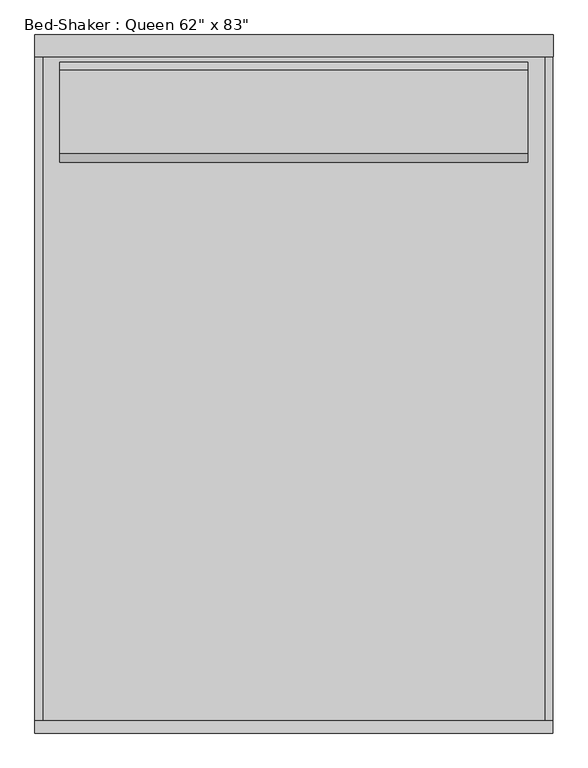
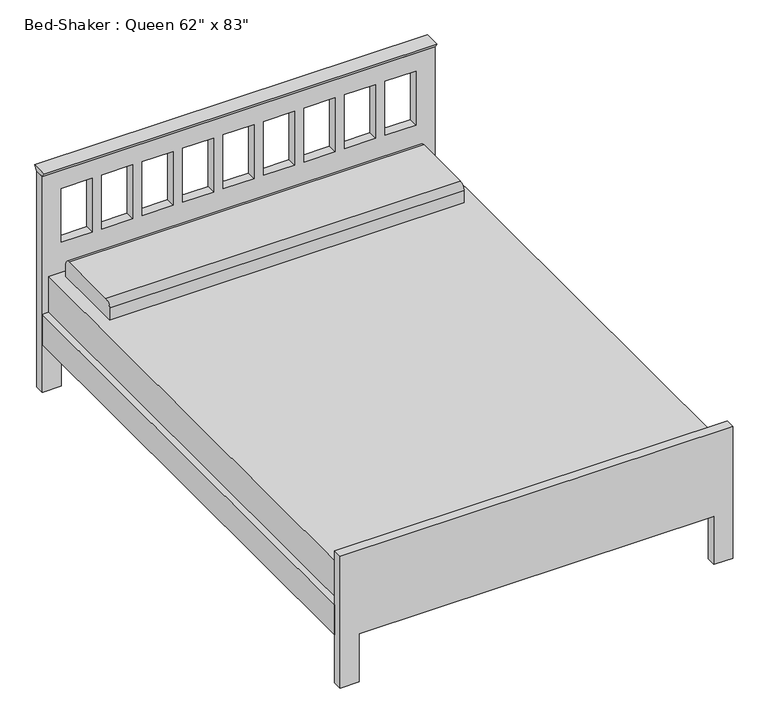
"""IFC4 building model written with IfcOpenShell, lengths in millimetres: furniture geometry."""

from ifc_helpers import new_model, si_unit, point, frame, frame_2d, origin, place, context, project, spatial, polyline, circle_curve, trimmed, segment, composite_curve, outline, extrude, source, transform, mapped, element, save


def furniture_35c09872(model_context):
    return source(origin(), model_context, "Body", "SweptSolid", [
        extrude(outline(polyline([(-38.1, 914.4), (-51.9545455, 933.45), (13.8545455, 933.45), (0.0, 914.4), (-38.1, 914.4)])), frame((-806.2365546, 0.0, 0.0), z_axis=(1.0, 0.0, 0.0), x_axis=(0.0, 1.0, 0.0)), (0.0, 0.0, 1.0), 1574.8533613),
        extrude(outline(composite_curve([segment(polyline([(-373.2486637, 482.6), (-373.2486637, 533.4)]), True, "CONTINUOUS"), segment(trimmed(circle_curve(frame_2d((-347.8486637, 533.4)), 25.4), [point((-373.2486637, 533.4))], [point((-347.8486637, 558.8))], False, "CARTESIAN"), True, "CONTINUOUS"), segment(polyline([(-347.8486637, 558.8), (-93.8486637, 558.8)]), True, "CONTINUOUS"), segment(trimmed(circle_curve(frame_2d((-93.8486637, 533.4)), 25.4), [point((-93.8486637, 558.8))], [point((-68.4486637, 533.4))], False, "CARTESIAN"), True, "CONTINUOUS"), segment(polyline([(-68.4486637, 533.4), (-68.4486637, 482.6), (-373.2486637, 482.6)]), True, "CONTINUOUS")], self_intersect=False)), frame((-730.25, 0.0, 0.0), z_axis=(1.0, 0.0, 0.0), x_axis=(0.0, 1.0, 0.0)), (0.0, 0.0, 1.0), 1422.4),
        extrude(outline(polyline([(742.95, -38.1), (742.95, -2070.1), (-781.05, -2070.1), (-781.05, -38.1), (742.95, -38.1)])), frame((0.0, 0.0, 228.6), z_axis=(0.0, 0.0, 1.0), x_axis=(1.0, 0.0, 0.0)), (0.0, 0.0, 1.0), 254.0),
        extrude(outline(polyline([(742.95, -2070.1), (742.95, -38.1), (768.35, -38.1), (768.35, -2070.1), (742.95, -2070.1)])), frame((0.0, 0.0, 203.0994861), z_axis=(0.0, 0.0, 1.0), x_axis=(1.0, 0.0, 0.0)), (0.0, 0.0, 1.0), 127.0),
        extrude(outline(polyline([(-806.45, -2070.1), (-806.45, -38.1), (-781.05, -38.1), (-781.05, -2070.1), (-806.45, -2070.1)])), frame((0.0, 0.0, 203.5755296), z_axis=(0.0, 0.0, 1.0), x_axis=(1.0, 0.0, 0.0)), (0.0, 0.0, 1.0), 127.0),
        extrude(outline(polyline([(0.0, -730.25), (203.2, -730.25), (203.2, 692.15), (0.0, 692.15), (0.0, 768.35), (558.8, 768.35), (558.8, -806.45), (0.0, -806.45), (0.0, -730.25)])), frame((0.0, -2108.2, 0.0), z_axis=(0.0, 1.0, 0.0), x_axis=(0.0, 0.0, 1.0)), (0.0, 0.0, 1.0), 38.1),
        extrude(outline(polyline([(914.4, 768.6168067), (914.4, -806.2365546), (0.0, -806.2365546), (0.0, -730.25), (203.2, -730.25), (203.2, 692.15), (0.0, 692.15), (0.0, 768.6168067), (914.4, 768.6168067)]), holes=[polyline([(838.2, -606.0722222), (609.6, -606.0722222), (609.6, -730.25), (838.2, -730.25), (838.2, -606.0722222)]), polyline([(838.2, -443.7944444), (609.6, -443.7944444), (609.6, -567.9722222), (838.2, -567.9722222), (838.2, -443.7944444)]), polyline([(838.2, -281.5166667), (609.6, -281.5166667), (609.6, -405.6944444), (838.2, -405.6944444), (838.2, -281.5166667)]), polyline([(838.2, -119.2388889), (609.6, -119.2388889), (609.6, -243.4166667), (838.2, -243.4166667), (838.2, -119.2388889)]), polyline([(838.2, 205.3166667), (609.6, 205.3166667), (609.6, 81.1388889), (838.2, 81.1388889), (838.2, 205.3166667)]), polyline([(838.2, 367.5944444), (609.6, 367.5944444), (609.6, 243.4166667), (838.2, 243.4166667), (838.2, 367.5944444)]), polyline([(838.2, 529.8722222), (609.6, 529.8722222), (609.6, 405.6944444), (838.2, 405.6944444), (838.2, 529.8722222)]), polyline([(838.2, 692.15), (609.6, 692.15), (609.6, 567.9722222), (838.2, 567.9722222), (838.2, 692.15)]), polyline([(838.2, 43.0388889), (609.6, 43.0388889), (609.6, -81.1388889), (838.2, -81.1388889), (838.2, 43.0388889)])]), frame((0.0, -38.1, 0.0), z_axis=(0.0, 1.0, 0.0), x_axis=(0.0, 0.0, 1.0)), (0.0, 0.0, 1.0), 38.1),
    ])


if __name__ == "__main__":
    model = new_model("IFC4")
    model_context = context("Model", 3, world=origin())
    ifc_project = project(units=[si_unit("LENGTHUNIT", "METRE", prefix="MILLI")], contexts=[model_context])
    site = spatial("IfcSite", under=ifc_project)
    building = spatial("IfcBuilding", under=site)
    placement = place(None, origin())
    furniture_shape = furniture_35c09872(model_context)
    element("IfcFurniture", 1, ObjectType="Bed-Shaker : Queen 62\" x 83\"", at=placement, inside=building, context=model_context, shape_type="MappedRepresentation", body=[
        mapped(furniture_shape, transform((0.0, 0.0, 0.0), x_axis=(1.0, 0.0, 0.0), y_axis=(0.0, 1.0, 0.0), z_axis=(0.0, 0.0, 1.0))),
    ])
    save(model, "model.ifc")

# Revit data of these elements
# Type "Bed-Shaker : Queen 62\" x 83\""
#   Assembly Code = "E2020200"
#   Length = 6' - 11"
#   Width = 5' - 2"
#   Frame Material = Birch
#   Mattress Material = Sash
#   Default Elevation = 0
# Element 1 (IfcFurniture, "Bed-Shaker : Queen 62\" x 83\"")
#   Materials on its faces: "Birch", "Sash"
# Materials
#   "Birch": class "Wood", colour RGB 224 178 126, transparency 0, Description = "Betula Alleghaniensis", Cost = 0
#   "Sash": class "Wood", colour RGB 224 178 126, transparency 0
